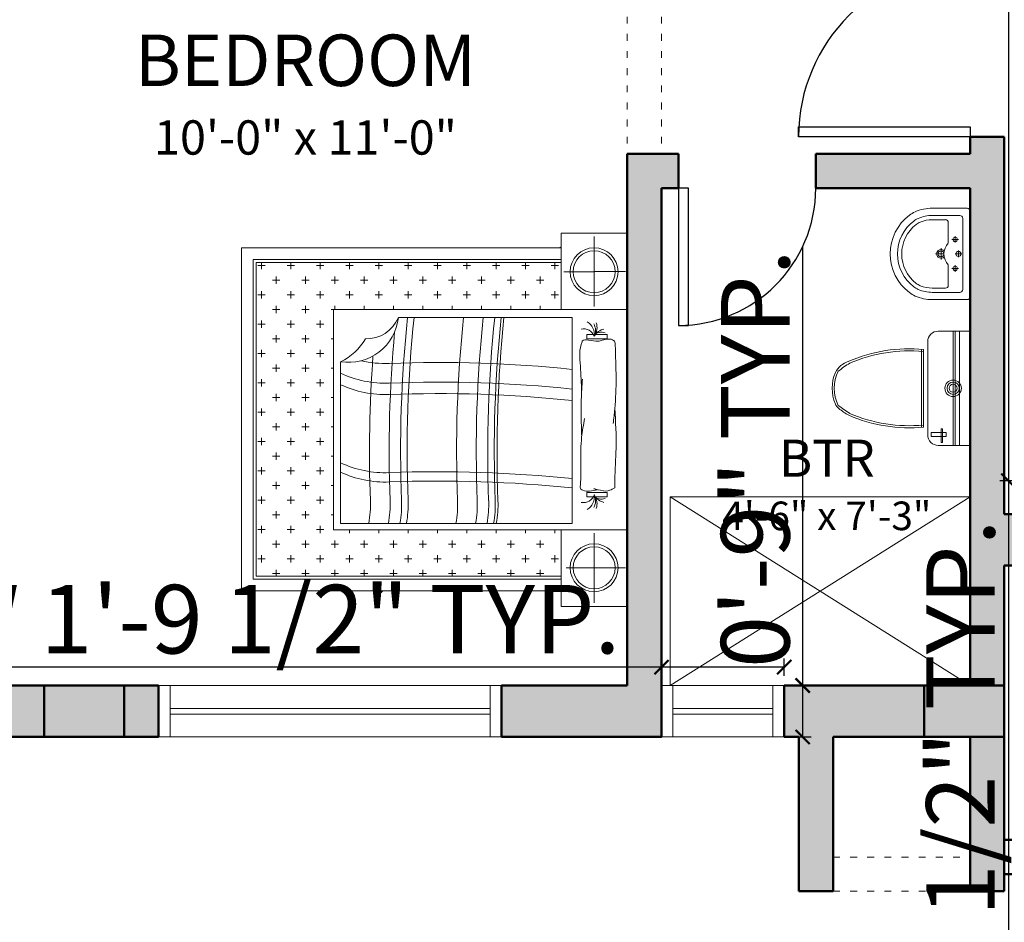
# Model space of a CAD drawing. Units: inches. Extents: x 375 to 1122, y 27 to 1069.
# Tile 3 of 155: x 494 to 667, y 155 to 313. Entities that reach past the tile are written whole.
import ezdxf

# ---------------------------------------------------------------- set-up
doc = ezdxf.new("R2010")
doc.units = ezdxf.units.IN
doc.linetypes.add('ACAD_ISO03W100', pattern=[30, 12, -18])
for name, color, linetype, lineweight in [('A-ANNO-DIMS', 2, 'Continuous', 18), ('A-AREA-IDEN', 7, 'Continuous', 18), ('A-COLS-PATT', 10, 'Continuous', 13), ('A-FLOR-FIXT', 55, 'Continuous', 18), ('A-WALL-OVHD', 77, 'ACAD_ISO03W100', 18), ('A-WALL-PATT', 252, 'Continuous', 13), ('Columns', 10, 'Continuous', 50), ('Doors', 150, 'Continuous', 25), ('Furniture', 30, 'Continuous', 18), ('Shower Areas', 53, 'Continuous', 18), ('Walls', 250, 'Continuous', 50), ('Windows', 122, 'Continuous', 18)]:
    doc.layers.add(name, color=color, linetype=linetype, lineweight=lineweight)
doc.styles.get("Standard").update_dxf_attribs({"font": 'arial.ttf'})
doc.dimstyles.new('ISO-25', dxfattribs={"dimtxt": 12, "dimasz": 2.5, "dimexe": 1.5, "dimexo": 1.5, "dimtad": 1, "dimdec": 1, "dimlunit": 3, "dimtxsty": 'Standard', "dimblk": 'ARCHTICK', "dimcen": 2.5, "dimadec": 0, "dimazin": 0, "dimtfac": 1, "dimtdec": 1, "dimtmove": 0, "dimatfit": 3, "dimfxl": 1.5, "dimfxlon": 1, "dimarcsym": 0})

# ---------------------------------------------------------------- blocks, each defined once
blk = doc.blocks.new('*U6')
for p, q in [((0, 0), (0, 4)), ((24, 0), (24, 4))]:
    blk.add_line(p, q)
blk.add_lwpolyline([(0, 0), (0, -24), (1.75, -24), (1.75, 0)], close=True)
blk.add_arc((0, 0), 24, 270, 0)
blk = doc.blocks.new('*U10')
for p, q in [((-30, 0), (-30, 4)), ((0, 0), (0, 4))]:
    blk.add_line(p, q)
blk.add_lwpolyline([(0, 0), (0, -30), (-1.75, -30), (-1.75, 0)], close=True)
blk.add_arc((0, 0), 30, 180, 270)
blk = doc.blocks.new('A$C52B64FF5')
for p, q in [((0.5216, 2.6276), (0, 2.6276)), ((0, 2.6276), (0, 2.1776)), ((0.5216, 2.1776), (0.5216, 2.6276)), ((2.0216, 2.6276), (0.5216, 2.6276)), ((0.5216, 2.6276), (0.5216, 0.6276)), ((2.5432, 2.6276), (2.0216, 2.6276)), ((2.0216, 0.6276), (2.0216, 2.6276)), ((2.0216, 2.6276), (2.0216, 2.1776)), ((2.5432, 2.1776), (2.5432, 2.6276)), ((0.2616, 2.4026), (0.2616, 2.6161)), ((2.2816, 2.4026), (2.2816, 2.6161)), ((0.721, 2.4927), (0.6917, 2.4927)), ((0.6917, 2.4927), (0.6917, 2.3531)), ((0.721, 2.3531), (0.721, 2.4927)), ((1.767, 2.3531), (1.767, 2.4927)), ((1.767, 2.4927), (1.7964, 2.4927)), ((1.7964, 2.4927), (1.7964, 2.3531)), ((0.2632, 2.4026), (0.0233, 2.4026)), ((0.0233, 2.4026), (0.4999, 2.4026)), ((0.2632, 2.1952), (0.2632, 2.4026)), ((0.6917, 2.3531), (0.721, 2.3531)), ((1.7964, 2.3531), (1.767, 2.3531)), ((2.5199, 2.4026), (2.0434, 2.4026)), ((2.2801, 2.2128), (2.2801, 2.4026)), ((2.2801, 2.4026), (2.5199, 2.4026)), ((0.5751, 1.0685), (0.5751, 2.2541)), ((0.5751, 2.2541), (1.9782, 2.2541)), ((1.9782, 2.2541), (1.9782, 0.6749)), ((0, 2.1776), (0.5216, 2.1776)), ((0.093, 2.1776), (0.1008, 2.1698)), ((0.1008, 0), (0.1008, 2.1776)), ((0.1808, 0.08), (0.1808, 2.1776)), ((0.2008, 0.1), (0.2008, 2.1776)), ((0.2197, 2.111), (0.2197, 2.161)), ((0.4197, 2.111), (0.4197, 2.161)), ((2.5432, 2.1776), (2.0216, 2.1776)), ((2.0216, 2.1776), (2.5432, 2.1776)), ((2.2197, 2.111), (2.2197, 2.161)), ((2.3374, 2.1776), (2.3374, 0.1)), ((2.3574, 2.1776), (2.3574, 0.08)), ((2.4374, 2.1776), (2.4374, 0)), ((0.2008, 2.136), (0.2447, 2.136)), ((0.3947, 2.136), (0.4447, 2.136)), ((2.0216, 2.136), (2.0447, 2.136)), ((2.1947, 2.136), (2.2447, 2.136)), ((0.2947, 2.036), (0.3447, 2.036)), ((0.3197, 2.011), (0.3197, 2.061)), ((0.4947, 2.036), (0.5216, 2.036)), ((0.5197, 2.011), (0.5197, 2.061)), ((2.0947, 2.036), (2.1447, 2.036)), ((2.1197, 2.011), (2.1197, 2.061)), ((2.2947, 2.036), (2.3374, 2.036)), ((2.3197, 2.011), (2.3197, 2.061)), ((0.2197, 1.911), (0.2197, 1.961)), ((0.4197, 1.911), (0.4197, 1.961)), ((2.2197, 1.911), (2.2197, 1.961)), ((0.2008, 1.936), (0.2447, 1.936)), ((0.3947, 1.936), (0.4447, 1.936)), ((2.0216, 1.936), (2.0447, 1.936)), ((2.1947, 1.936), (2.2447, 1.936)), ((0.2947, 1.836), (0.3447, 1.836)), ((0.3197, 1.811), (0.3197, 1.861)), ((0.4947, 1.836), (0.5216, 1.836)), ((0.5197, 1.811), (0.5197, 1.861)), ((2.0947, 1.836), (2.1447, 1.836)), ((2.1197, 1.811), (2.1197, 1.861)), ((2.2947, 1.836), (2.3374, 1.836)), ((2.3197, 1.811), (2.3197, 1.861)), ((0.2197, 1.711), (0.2197, 1.761)), ((0.4197, 1.711), (0.4197, 1.761)), ((2.2197, 1.711), (2.2197, 1.761)), ((0.2008, 1.736), (0.2447, 1.736)), ((0.3947, 1.736), (0.4447, 1.736)), ((2.0216, 1.736), (2.0447, 1.736)), ((2.1947, 1.736), (2.2447, 1.736)), ((0.2947, 1.636), (0.3447, 1.636)), ((0.3197, 1.611), (0.3197, 1.661)), ((0.4947, 1.636), (0.5216, 1.636)), ((0.5197, 1.611), (0.5197, 1.661)), ((2.0947, 1.636), (2.1447, 1.636)), ((2.1197, 1.611), (2.1197, 1.661)), ((2.2947, 1.636), (2.3374, 1.636)), ((2.3197, 1.611), (2.3197, 1.661)), ((0.2197, 1.511), (0.2197, 1.561)), ((0.4197, 1.511), (0.4197, 1.561)), ((2.2197, 1.511), (2.2197, 1.561)), ((0.2008, 1.536), (0.2447, 1.536)), ((0.3947, 1.536), (0.4447, 1.536)), ((2.0216, 1.536), (2.0447, 1.536)), ((2.1947, 1.536), (2.2447, 1.536)), ((0.2947, 1.436), (0.3447, 1.436)), ((0.3197, 1.411), (0.3197, 1.461)), ((0.4947, 1.436), (0.5216, 1.436)), ((0.5197, 1.411), (0.5197, 1.461)), ((2.0947, 1.436), (2.1447, 1.436)), ((2.1197, 1.411), (2.1197, 1.461)), ((2.2947, 1.436), (2.3374, 1.436)), ((2.3197, 1.411), (2.3197, 1.461)), ((0.2197, 1.311), (0.2197, 1.361)), ((0.4197, 1.311), (0.4197, 1.361)), ((2.2197, 1.311), (2.2197, 1.361)), ((0.2008, 1.336), (0.2447, 1.336)), ((0.3947, 1.336), (0.4447, 1.336)), ((2.0216, 1.336), (2.0447, 1.336)), ((2.1947, 1.336), (2.2447, 1.336)), ((0.2947, 1.236), (0.3447, 1.236)), ((0.3197, 1.211), (0.3197, 1.261)), ((0.4947, 1.236), (0.5216, 1.236)), ((0.5197, 1.211), (0.5197, 1.261)), ((2.0947, 1.236), (2.1447, 1.236)), ((2.1197, 1.211), (2.1197, 1.261)), ((2.2947, 1.236), (2.3374, 1.236)), ((2.3197, 1.211), (2.3197, 1.261)), ((0.2197, 1.111), (0.2197, 1.161)), ((0.4197, 1.111), (0.4197, 1.161)), ((2.2197, 1.111), (2.2197, 1.161)), ((0.2008, 1.136), (0.2447, 1.136)), ((0.3947, 1.136), (0.4447, 1.136)), ((2.0216, 1.136), (2.0447, 1.136)), ((2.1947, 1.136), (2.2447, 1.136)), ((0.2947, 1.036), (0.3447, 1.036)), ((0.3197, 1.011), (0.3197, 1.061)), ((0.4947, 1.036), (0.5216, 1.036)), ((0.5197, 1.011), (0.5197, 1.061)), ((2.0947, 1.036), (2.1447, 1.036)), ((2.1197, 1.011), (2.1197, 1.061)), ((2.2947, 1.036), (2.3374, 1.036)), ((2.3197, 1.011), (2.3197, 1.061)), ((0.2197, 0.911), (0.2197, 0.961)), ((0.4197, 0.911), (0.4197, 0.961)), ((2.2197, 0.911), (2.2197, 0.961)), ((2.4374, 0.9617), (2.4642, 0.935)), ((0.2008, 0.936), (0.2447, 0.936)), ((0.3947, 0.936), (0.4447, 0.936)), ((2.0216, 0.936), (2.0447, 0.936)), ((2.1947, 0.936), (2.2447, 0.936)), ((0.2947, 0.836), (0.3447, 0.836)), ((0.3197, 0.811), (0.3197, 0.861)), ((0.4947, 0.836), (0.5216, 0.836)), ((0.5197, 0.811), (0.5197, 0.861)), ((2.0947, 0.836), (2.1447, 0.836)), ((2.1197, 0.811), (2.1197, 0.861)), ((2.2947, 0.836), (2.3374, 0.836)), ((2.3197, 0.811), (2.3197, 0.861)), ((0.2197, 0.711), (0.2197, 0.761)), ((0.4197, 0.711), (0.4197, 0.761)), ((2.2197, 0.711), (2.2197, 0.761)), ((0.2008, 0.736), (0.2447, 0.736)), ((0.3947, 0.736), (0.4447, 0.736)), ((1.9782, 0.6749), (0.8764, 0.6749)), ((2.0216, 0.736), (2.0447, 0.736)), ((2.1947, 0.736), (2.2447, 0.736)), ((0.2947, 0.636), (0.3447, 0.636)), ((0.3197, 0.611), (0.3197, 0.661)), ((0.4947, 0.636), (0.5216, 0.636)), ((0.5197, 0.611), (0.5197, 0.661)), ((0.5216, 0.6276), (2.0216, 0.6276)), ((0.7197, 0.611), (0.7197, 0.6276)), ((0.9197, 0.611), (0.9197, 0.6276)), ((1.1197, 0.611), (1.1197, 0.6276)), ((1.3197, 0.611), (1.3197, 0.6276)), ((1.5197, 0.611), (1.5197, 0.6276)), ((1.7197, 0.611), (1.7197, 0.6276)), ((1.9197, 0.611), (1.9197, 0.6276)), ((2.0947, 0.636), (2.1447, 0.636)), ((2.1197, 0.611), (2.1197, 0.661)), ((2.2947, 0.636), (2.3374, 0.636)), ((2.3197, 0.611), (2.3197, 0.661)), ((0.2197, 0.511), (0.2197, 0.561)), ((0.4197, 0.511), (0.4197, 0.561)), ((0.6197, 0.511), (0.6197, 0.561)), ((0.8197, 0.511), (0.8197, 0.561)), ((1.0197, 0.511), (1.0197, 0.561)), ((1.2197, 0.511), (1.2197, 0.561)), ((1.4197, 0.511), (1.4197, 0.561)), ((1.6197, 0.511), (1.6197, 0.561)), ((1.8197, 0.511), (1.8197, 0.561)), ((2.0197, 0.511), (2.0197, 0.561)), ((2.2197, 0.511), (2.2197, 0.561)), ((0.2008, 0.536), (0.2447, 0.536)), ((0.3947, 0.536), (0.4447, 0.536)), ((0.5947, 0.536), (0.6447, 0.536)), ((0.7947, 0.536), (0.8447, 0.536)), ((0.9947, 0.536), (1.0447, 0.536)), ((1.1947, 0.536), (1.2447, 0.536)), ((1.3947, 0.536), (1.4447, 0.536)), ((1.5947, 0.536), (1.6447, 0.536)), ((1.7947, 0.536), (1.8447, 0.536)), ((1.9947, 0.536), (2.0447, 0.536)), ((2.1947, 0.536), (2.2447, 0.536)), ((0.2947, 0.436), (0.3447, 0.436)), ((0.3197, 0.411), (0.3197, 0.461)), ((0.4947, 0.436), (0.5447, 0.436)), ((0.5197, 0.411), (0.5197, 0.461)), ((0.6947, 0.436), (0.7447, 0.436)), ((0.7197, 0.411), (0.7197, 0.461)), ((0.8947, 0.436), (0.9447, 0.436)), ((0.9197, 0.411), (0.9197, 0.461)), ((1.0947, 0.436), (1.1447, 0.436)), ((1.1197, 0.411), (1.1197, 0.461)), ((1.2947, 0.436), (1.3447, 0.436)), ((1.3197, 0.411), (1.3197, 0.461)), ((1.4947, 0.436), (1.5447, 0.436)), ((1.5197, 0.411), (1.5197, 0.461)), ((1.6947, 0.436), (1.7447, 0.436)), ((1.7197, 0.411), (1.7197, 0.461)), ((1.8947, 0.436), (1.9447, 0.436)), ((1.9197, 0.411), (1.9197, 0.461)), ((2.0947, 0.436), (2.1447, 0.436)), ((2.1197, 0.411), (2.1197, 0.461)), ((2.2947, 0.436), (2.3374, 0.436)), ((2.3197, 0.411), (2.3197, 0.461)), ((0.2008, 0.336), (0.2447, 0.336)), ((0.2197, 0.311), (0.2197, 0.361)), ((0.3947, 0.336), (0.4447, 0.336)), ((0.4197, 0.311), (0.4197, 0.361)), ((0.5947, 0.336), (0.6447, 0.336)), ((0.6197, 0.311), (0.6197, 0.361)), ((0.7947, 0.336), (0.8447, 0.336)), ((0.8197, 0.311), (0.8197, 0.361)), ((0.9947, 0.336), (1.0447, 0.336)), ((1.0197, 0.311), (1.0197, 0.361)), ((1.1947, 0.336), (1.2447, 0.336)), ((1.2197, 0.311), (1.2197, 0.361)), ((1.3947, 0.336), (1.4447, 0.336)), ((1.4197, 0.311), (1.4197, 0.361)), ((1.5947, 0.336), (1.6447, 0.336)), ((1.6197, 0.311), (1.6197, 0.361)), ((1.7947, 0.336), (1.8447, 0.336)), ((1.8197, 0.311), (1.8197, 0.361)), ((1.9947, 0.336), (2.0447, 0.336)), ((2.0197, 0.311), (2.0197, 0.361)), ((2.1947, 0.336), (2.2447, 0.336)), ((2.2197, 0.311), (2.2197, 0.361)), ((0.2947, 0.236), (0.3447, 0.236)), ((0.3197, 0.211), (0.3197, 0.261)), ((0.4947, 0.236), (0.5447, 0.236)), ((0.5197, 0.211), (0.5197, 0.261)), ((0.6947, 0.236), (0.7447, 0.236)), ((0.7197, 0.211), (0.7197, 0.261)), ((0.8947, 0.236), (0.9447, 0.236)), ((0.9197, 0.211), (0.9197, 0.261)), ((1.0947, 0.236), (1.1447, 0.236)), ((1.1197, 0.211), (1.1197, 0.261)), ((1.2947, 0.236), (1.3447, 0.236)), ((1.3197, 0.211), (1.3197, 0.261)), ((1.4947, 0.236), (1.5447, 0.236)), ((1.5197, 0.211), (1.5197, 0.261)), ((1.6947, 0.236), (1.7447, 0.236)), ((1.7197, 0.211), (1.7197, 0.261)), ((1.8947, 0.236), (1.9447, 0.236)), ((1.9197, 0.211), (1.9197, 0.261)), ((2.0947, 0.236), (2.1447, 0.236)), ((2.1197, 0.211), (2.1197, 0.261)), ((2.2947, 0.236), (2.3374, 0.236)), ((2.3197, 0.211), (2.3197, 0.261)), ((0.2008, 0.136), (0.2447, 0.136)), ((0.2197, 0.111), (0.2197, 0.161)), ((0.3947, 0.136), (0.4447, 0.136)), ((0.4197, 0.111), (0.4197, 0.161)), ((0.5947, 0.136), (0.6447, 0.136)), ((0.6197, 0.111), (0.6197, 0.161)), ((0.7947, 0.136), (0.8447, 0.136)), ((0.8197, 0.111), (0.8197, 0.161)), ((0.9947, 0.136), (1.0447, 0.136)), ((1.0197, 0.111), (1.0197, 0.161)), ((1.1947, 0.136), (1.2447, 0.136)), ((1.2197, 0.111), (1.2197, 0.161)), ((1.3947, 0.136), (1.4447, 0.136)), ((1.4197, 0.111), (1.4197, 0.161)), ((1.5947, 0.136), (1.6447, 0.136)), ((1.6197, 0.111), (1.6197, 0.161)), ((1.7947, 0.136), (1.8447, 0.136)), ((1.8197, 0.111), (1.8197, 0.161)), ((1.9947, 0.136), (2.0447, 0.136)), ((2.0197, 0.111), (2.0197, 0.161)), ((2.1947, 0.136), (2.2447, 0.136)), ((2.2197, 0.111), (2.2197, 0.161)), ((2.3574, 0.08), (0.1808, 0.08)), ((2.3374, 0.1), (0.2008, 0.1)), ((2.4374, 0), (0.1008, 0))]:
    blk.add_line(p, q)
for centre, radius in [((0.2632, 2.4026), 0.1631), ((2.2801, 2.4026), 0.1631), ((0.2632, 2.4026), 0.1431), ((2.2801, 2.4026), 0.1431)]:
    blk.add_circle(centre, radius)
for centre, radius, start, end in [((0.6442, 2.3154), 0.1072, 59.2174, 107.24009), ((0.7523, 2.4916), 0.1013, 192.77399, 239.2386), ((0.7566, 2.4523), 0.0808, 161.45592, 221.5545), ((1.7358, 2.4916), 0.1013, 300.7614, 347.22601), ((1.8439, 2.3154), 0.1072, 72.75991, 120.7826), ((1.7315, 2.4523), 0.0808, 318.4455, 18.54408), ((0.6895, 2.3063), 0.098, 80.94857, 149.48786), ((0.6646, 2.3215), 0.0913, 67.83977, 120.48585), ((0.7294, 2.33), 0.0776, 109.26419, 192.26691), ((1.7587, 2.33), 0.0776, 347.73309, 73.88358), ((1.7986, 2.3063), 0.098, 30.51214, 99.05143), ((1.8235, 2.3215), 0.0913, 59.51415, 112.16023), ((9.7293, 1.3409), 8.8479, 174.07538, 182.16616), ((9.8633, 1.3409), 8.8479, 174.07538, 182.16616), ((9.9414, 1.3409), 8.8479, 174.07538, 182.16616), ((10.4736, 1.3409), 8.8479, 174.07538, 182.16616), ((10.5369, 1.3409), 8.8479, 174.07538, 182.16616), ((1.4884, 10.5889), 8.8479, 264.07538, 272.16616), ((1.4884, 10.5702), 8.8479, 264.07538, 272.16616), ((1.85, 1.0282), 0.7196, 79.7409, 92.16616), ((1.4884, 10.5256), 8.8479, 264.07538, 272.16616), ((1.85, 1.0096), 0.7196, 79.7409, 92.16616), ((1.85, 0.965), 0.7196, 79.7409, 92.16616), ((1.4884, 10.4474), 8.8479, 264.07538, 272.16616), ((1.85, 0.8868), 0.7196, 79.7409, 92.16616), ((1.4884, 10.3135), 8.8479, 264.07538, 272.16616), ((1.85, 0.7528), 0.7196, 79.7409, 92.16616), ((1.4884, 9.9764), 8.8479, 264.07538, 272.16616), ((1.4884, 9.9317), 8.8479, 264.07538, 272.16616), ((1.85, 0.4158), 0.7196, 79.7409, 92.16616), ((1.85, 0.3711), 0.7196, 79.7409, 92.16616), ((0.4865, 0.8516), 0.2343, 358.03681, 67.7864), ((0.5391, 0.7288), 0.3416, 350.92672, 83.95649), ((1.4884, 9.8536), 8.8479, 264.70583, 272.16616), ((1.85, 0.293), 0.7196, 79.7409, 92.16616), ((0.1687, 0.9792), 0.7196, 346.86533, 2.16616), ((0.3027, 0.9792), 0.7196, 334.98359, 2.16616), ((0.3808, 0.9792), 0.7196, 334.98359, 2.16616), ((0.913, 0.9792), 0.7196, 334.98359, 2.16616), ((0.9763, 0.9792), 0.7196, 334.98359, 2.16616), ((1.4884, 9.7196), 8.8479, 265.77852, 272.16616), ((1.85, 0.159), 0.7196, 79.7409, 92.16616), ((0.5285, 0.5098), 0.3852, 25.3912, 60.06861)]:
    blk.add_arc(centre, radius, start, end)
for points, knots in [([(0.7373, 2.4293), (0.7344, 2.4386), (0.7239, 2.472), (0.715, 2.518), (0.7414, 2.5459), (0.9088, 2.5514), (1.0864, 2.5586), (1.2642, 2.5365), (1.2976, 2.5323)], [0, 0, 0, 0, 0.0298664, 0.1071619, 0.1152509, 0.1416099, 0.5761797, 0.6768951, 0.6768951, 0.6768951, 0.6768951]), ([(1.1947, 2.5438), (1.2853, 2.549), (1.4483, 2.5585), (1.6283, 2.5432), (1.7179, 2.5437), (1.7351, 2.5438)], [0, 0, 0, 0, 0.2717358, 0.4891854, 0.5406465, 0.5406465, 0.5406465, 0.5406465]), ([(1.7351, 2.5438), (1.7416, 2.5321), (1.759, 2.5014), (1.7583, 2.4623), (1.7348, 2.3817), (1.7455, 2.4145), (1.7494, 2.4265)], [0, 0, 0, 0, 0.0383771, 0.1013156, 0.1484959, 0.1756343, 0.1756343, 0.1756343, 0.1756343]), ([(1.0802, 2.3175), (1.0225, 2.3155), (0.9099, 2.3116), (0.7905, 2.2985), (0.7234, 2.3279), (0.7309, 2.3766), (0.7348, 2.4091), (0.7373, 2.4293)], [0, 0, 0, 0, 0.1744349, 0.3406483, 0.347042, 0.3874998, 0.4538558, 0.4538558, 0.4538558, 0.4538558]), ([(1.7494, 2.4265), (1.7531, 2.4084), (1.7601, 2.3751), (1.7573, 2.3363), (1.7437, 2.3065), (1.6676, 2.315), (1.559, 2.3108), (1.4028, 2.3119), (1.305, 2.3301), (1.2633, 2.3378)], [0, 0, 0, 0, 0.0550284, 0.1011576, 0.1178362, 0.1437253, 0.3009935, 0.4726259, 0.6000038, 0.6000038, 0.6000038, 0.6000038]), ([(1.3748, 2.3178), (1.2947, 2.315), (1.1678, 2.3105), (1.0413, 2.32), (0.9946, 2.3235)], [0, 0, 0, 0, 0.2401688, 0.38052, 0.38052, 0.38052, 0.38052])]:
    blk.add_open_spline(points, degree=3, knots=knots)
blk = doc.blocks.new('A$C00C51FE0')
at = {"ltscale": 2}
for p, q in [((1.85, 7.41), (18.15, 7.41)), ((16.79, 8.49), (3.21, 8.49)), ((16.79, 8.12), (3.21, 8.12)), ((0, 0), (0, 5.56)), ((1.59, 4.18), (1.59, 6.81)), ((1.59, 6.81), (2.25, 6.81)), ((2.25, 6.81), (2.25, 4.18)), ((20, 5.56), (20, 0)), ((0.5, 4.84), (0.5, 5.06)), ((0.5, 5.06), (2.91, 5.06)), ((2.91, 4.84), (0.5, 4.84)), ((2.25, 4.18), (1.59, 4.18)), ((2.91, 5.06), (2.91, 4.84)), ((20, 2.96), (0, 2.96)), ((20, 2.59), (0, 2.59)), ((20, 1.85), (0, 1.85)), ((20, 0), (0, 0))]:
    blk.add_line(p, q, dxfattribs=at)
for radius in [1.44, 1.07, 0.698]:
    blk.add_circle((10, 2.96), radius, dxfattribs=at)
for centre, radius, start, end in [((10, 17.03), 7.1, 67.0801, 112.9199), ((22.68, 10.69), 20.34, 142.816, 148.8373), ((22.68, 10.69), 19.97, 141.7352, 148.8373), ((7.96, 21.86), 1.85, 112.9199, 142.816), ((10, 17.03), 6.73, 63.5839, 116.4161), ((11.04, 20.15), 3.83, 16.1902, 63.2078), ((-2.68, 10.69), 19.97, 31.1627, 38.2648), ((29.69, 10.65), 26.6, 156.5869, 185.4494), ((29.69, 10.65), 26.23, 156.5869, 185.4494), ((-9.69, 10.65), 26.23, 354.5506, 23.4131), ((-9.69, 10.65), 26.6, 354.5506, 23.4131), ((1.85, 5.56), 1.85, 90, 180), ((18.15, 5.56), 1.85, 0, 90)]:
    blk.add_arc(centre, radius, start, end, dxfattribs=at)
blk = doc.blocks.new('WINDOW-21_5IN')
for p, q in [((4, 2), (4, 19.5)), ((5, 2), (5, 19.5))]:
    blk.add_line(p, q)
blk.add_lwpolyline([(0, 0), (9, 0), (9, 21.5), (0, 21.5)], close=True)
for points in [[(9, 19.5), (0, 19.5)], [(0, 2), (9, 2)]]:
    blk.add_lwpolyline(points)
blk = doc.blocks.new('WINDOW-60IN')
for p, q in [((58, 5), (2, 5)), ((58, 4), (2, 4))]:
    blk.add_line(p, q)
blk.add_lwpolyline([(60, 0), (0, 0), (0, 9), (60, 9)], close=True)
for points in [[(2, 0), (2, 9)], [(58, 9), (58, 0)]]:
    blk.add_lwpolyline(points)
blk = doc.blocks.new('LAVATORY-16IN')
for p, q in [((1.27, 7.37), (1.27, 12.19)), ((1.78, 12.7), (14.22, 12.7)), ((8, 11.37), (8, 12.51)), ((14.73, 12.19), (14.73, 7.37)), ((4.89, 11.37), (6.03, 11.37)), ((5.46, 10.79), (5.46, 11.94)), ((7.43, 11.94), (8.57, 11.94)), ((9.97, 11.37), (11.11, 11.37)), ((10.54, 10.79), (10.54, 11.94)), ((2.01, 7.37), (2.01, 9.65)), ((2.51, 10.16), (6.08, 10.16)), ((7.02, 8.89), (8.98, 8.89)), ((8, 7.91), (8, 9.4)), ((9.91, 10.16), (13.49, 10.16)), ((13.99, 9.65), (13.99, 7.37))]:
    blk.add_line(p, q)
blk.add_lwpolyline([(0.51, 13.97), (15.49, 13.97, -0.414214), (16, 13.46), (16, 7.37, -0.104704), (15.37, 4.36, -0.038376), (14.78, 3.36, -0.495903), (1.22, 3.36, -0.038376), (0.63, 4.36, -0.104704), (0, 7.37), (0, 13.46, -0.414214)], format="xyb", close=True)
for points in [[(1.27, 7.37, 0.102694), (1.78, 4.92, 0.037256), (2.25, 4.11, 0.085618)], [(2.01, 7.37, 0.101044), (2.44, 5.24, 0.036381), (2.84, 4.54, 0.084644)], [(13.16, 4.54, 0.036381), (13.56, 5.24, 0.101044), (13.99, 7.37, 0.11083)], [(13.75, 4.11, 0.037256), (14.22, 4.92, 0.102694), (14.73, 7.37, 0.111333)]]:
    blk.add_lwpolyline(points, format="xyb")
for centre, radius in [((8, 11.94), 0.444), ((5.46, 11.37), 0.381), ((10.54, 11.37), 0.381), ((8, 8.89), 0.508)]:
    blk.add_circle(centre, radius)
for centre, radius, start, end in [((1.78, 12.19), 0.508, 90, 180), ((14.22, 12.19), 0.508, 0, 90), ((2.51, 9.65), 0.508, 90, 180), ((7.99, 12.19), 2.79, 226.6581, 313.3419), ((8, 8.89), 0.762, 133.135, 47.0367), ((13.49, 9.65), 0.508, 0, 90), ((8, 8.52), 7.25, 217.471, 322.529), ((8, 8.52), 6.51, 217.6433, 322.3567)]:
    blk.add_arc(centre, radius, start, end)
blk = doc.blocks.new('COLUMN-14X9IN')
blk.add_lwpolyline([(0, 0), (14, 0), (14, 9), (0, 9)], close=True)
blk = doc.blocks.new('SHOWER-PAN-52_5X33IN')
for p, q in [((0, 33), (52.5, 0)), ((52.5, 33), (0, 0))]:
    blk.add_line(p, q)
blk.add_lwpolyline([(0, 0), (52.5, 0), (52.5, 33), (0, 33)], close=True)
blk = doc.blocks.new('_ArchTick')
at = {"color": 0, "linetype": 'ByBlock', "const_width": 0.15}
blk.add_lwpolyline([(-0.5, -0.5), (0.5, 0.5)], dxfattribs=at)
blk = doc.blocks.new('*D49')
at = {"layer": 'A-ANNO-DIMS', "color": 0, "lineweight": -2, "transparency": 16777216}
for p, q in [((606.51, 198.25), (606.51, 201.25)), ((628.01, 198.25), (628.01, 201.25)), ((606.51, 199.75), (374.6, 199.75)), ((628.01, 199.75), (606.51, 199.75))]:
    blk.add_line(p, q, dxfattribs=at)
at = {"layer": 'Defpoints', "color": 0, "transparency": 16777216}
for p in [(606.51, 199.75), (606.51, 196.53), (628.01, 196.53)]:
    blk.add_point(p, dxfattribs=at)
at = {"layer": 'A-ANNO-DIMS', "color": 0, "lineweight": -2, "transparency": 16777216, "xscale": 2.5, "yscale": 2.5, "zscale": 2.5, "rotation": 180}
blk.add_blockref('_ArchTick', (606.51, 199.75), dxfattribs=at)
at = {"layer": 'A-ANNO-DIMS', "color": 0, "lineweight": -2, "transparency": 16777216, "xscale": 2.5, "yscale": 2.5, "zscale": 2.5}
blk.add_blockref('_ArchTick', (628.01, 199.75), dxfattribs=at)
at = {"layer": 'A-ANNO-DIMS', "color": 0, "transparency": 16777216, "insert": (489.3, 206.59), "char_height": 12, "attachment_point": 5}
blk.add_mtext('BATH WINDOW 1\'-9 1/2" TYP.', dxfattribs=at)
blk = doc.blocks.new('*D50')
at = {"layer": 'A-ANNO-DIMS', "color": 0, "lineweight": -2, "transparency": 16777216}
for p, q in [((631.23, 196.53), (631.23, 273.42)), ((629.73, 196.53), (632.73, 196.53)), ((631.23, 187.53), (631.23, 196.53)), ((629.73, 187.53), (632.73, 187.53))]:
    blk.add_line(p, q, dxfattribs=at)
at = {"layer": 'Defpoints', "color": 0, "transparency": 16777216}
for p in [(628.01, 196.53), (631.23, 196.53), (628.01, 187.53)]:
    blk.add_point(p, dxfattribs=at)
at = {"layer": 'A-ANNO-DIMS', "color": 0, "lineweight": -2, "transparency": 16777216, "xscale": 2.5, "yscale": 2.5, "zscale": 2.5}
for p, rotation in [((631.23, 196.53), 90), ((631.23, 187.53), 270)]:
    blk.add_blockref('_ArchTick', p, dxfattribs=dict(at, rotation=rotation))
at = {"layer": 'A-ANNO-DIMS', "color": 0, "transparency": 16777216, "insert": (624.48, 236.23), "char_height": 12, "attachment_point": 5, "rotation": 90}
blk.add_mtext('0\'-9" TYP.', dxfattribs=at)
blk = doc.blocks.new('*D59')
at = {"layer": 'A-ANNO-DIMS', "color": 0, "lineweight": -2, "transparency": 16777216}
for p, q in [((668.72, 346.85), (665.72, 346.85)), ((667.22, 346.85), (667.22, 232.35)), ((668.72, 232.35), (665.72, 232.35)), ((667.22, 232.35), (667.22, 27.5))]:
    blk.add_line(p, q, dxfattribs=at)
at = {"layer": 'Defpoints', "color": 0, "transparency": 16777216}
for p in [(684.39, 346.85), (667.22, 232.35), (684.39, 232.35)]:
    blk.add_point(p, dxfattribs=at)
at = {"layer": 'A-ANNO-DIMS', "color": 0, "lineweight": -2, "transparency": 16777216, "xscale": 2.5, "yscale": 2.5, "zscale": 2.5}
for p, rotation in [((667.22, 346.85), 90), ((667.22, 232.35), 270)]:
    blk.add_blockref('_ArchTick', p, dxfattribs=dict(at, rotation=rotation))
at = {"layer": 'A-ANNO-DIMS', "color": 0, "transparency": 16777216, "insert": (660.39, 128.67), "char_height": 12, "attachment_point": 5, "rotation": 90}
blk.add_mtext('DINING SET 9\'-6 1/2" TYP.', dxfattribs=at)
blk = doc.blocks.new('*D81')
at = {"layer": 'A-ANNO-DIMS', "color": 0, "lineweight": -2, "transparency": 16777216}
for p, q in [((444.51, 117.53), (444.51, 114.53)), ((989.01, 117.53), (989.01, 114.53)), ((444.51, 116.03), (989.01, 116.03))]:
    blk.add_line(p, q, dxfattribs=at)
at = {"layer": 'Defpoints', "color": 0, "transparency": 16777216}
for p in [(444.51, 187.53), (989.01, 187.53), (989.01, 116.03)]:
    blk.add_point(p, dxfattribs=at)
at = {"layer": 'A-ANNO-DIMS', "color": 0, "lineweight": -2, "transparency": 16777216, "xscale": 2.5, "yscale": 2.5, "zscale": 2.5, "rotation": 180}
blk.add_blockref('_ArchTick', (444.51, 116.03), dxfattribs=at)
at = {"layer": 'A-ANNO-DIMS', "color": 0, "lineweight": -2, "transparency": 16777216, "xscale": 2.5, "yscale": 2.5, "zscale": 2.5}
blk.add_blockref('_ArchTick', (989.01, 116.03), dxfattribs=at)
at = {"layer": 'A-ANNO-DIMS', "color": 0, "transparency": 16777216, "insert": (716.76, 122.86), "char_height": 12, "attachment_point": 5}
blk.add_mtext('45\'-4 1/2"', dxfattribs=at)
blk = doc.blocks.new('*D82')
at = {"layer": 'A-ANNO-DIMS', "color": 0, "lineweight": -2, "transparency": 16777216}
for p, q in [((401.51, 1009.53), (398.51, 1009.53)), ((400.01, 160.53), (400.01, 1009.53)), ((401.51, 160.53), (398.51, 160.53))]:
    blk.add_line(p, q, dxfattribs=at)
at = {"layer": 'Defpoints', "color": 0, "transparency": 16777216}
for p in [(400.01, 1009.53), (630.53, 1009.53), (630.53, 160.53)]:
    blk.add_point(p, dxfattribs=at)
at = {"layer": 'A-ANNO-DIMS', "color": 0, "lineweight": -2, "transparency": 16777216, "xscale": 2.5, "yscale": 2.5, "zscale": 2.5}
for p, rotation in [((400.01, 1009.53), 90), ((400.01, 160.53), 270)]:
    blk.add_blockref('_ArchTick', p, dxfattribs=dict(at, rotation=rotation))
at = {"layer": 'A-ANNO-DIMS', "color": 0, "transparency": 16777216, "insert": (393.26, 585.03), "char_height": 12, "attachment_point": 5, "rotation": 90}
blk.add_mtext('70\'-9"', dxfattribs=at)

msp = doc.modelspace()

# ---------------------------------------------------------------- hatches: boundary and pattern name
at = {"layer": 'A-COLS-PATT'}
h = msp.add_hatch(color=256, dxfattribs=at)
h.dxf.hatch_style = 1
h.paths.add_polyline_path([(512.51, 982.53), (498.51, 982.53), (498.51, 973.53), (512.51, 973.53)])
h.paths.add_polyline_path([(666.51, 982.53), (652.51, 982.53), (652.51, 973.53), (666.51, 973.53)])
h.paths.add_polyline_path([(802.01, 982.53), (788.01, 982.53), (788.01, 973.53), (802.01, 973.53)])
h.paths.add_polyline_path([(932.01, 982.53), (918.01, 982.53), (918.01, 973.53), (932.01, 973.53)])
h.paths.add_polyline_path([(507.51, 841.53), (498.51, 841.53), (498.51, 827.53), (507.51, 827.53)])
h.paths.add_polyline_path([(666.51, 844.53), (652.51, 844.53), (652.51, 835.53), (666.51, 835.53)])
h.paths.add_polyline_path([(802.01, 814.53), (788.01, 814.53), (788.01, 805.53), (802.01, 805.53)])
h.paths.add_polyline_path([(932.01, 814.53), (918.01, 814.53), (918.01, 805.53), (932.01, 805.53)])
h.paths.add_polyline_path([(507.51, 719.53), (498.51, 719.53), (498.51, 705.53), (507.51, 705.53)])
h.paths.add_polyline_path([(731.01, 676.53), (722.01, 676.53), (722.01, 662.53), (731.01, 662.53)])
h.paths.add_polyline_path([(802.01, 676.53), (788.01, 676.53), (788.01, 667.53), (802.01, 667.53)])
h.paths.add_polyline_path([(932.01, 676.53), (918.01, 676.53), (918.01, 667.53), (932.01, 667.53)])
h.paths.add_polyline_path([(932.01, 583.53), (918.01, 583.53), (918.01, 574.53), (932.01, 574.53)])
h.paths.add_polyline_path([(868.01, 583.53), (854.01, 583.53), (854.01, 574.53), (868.01, 574.53)])
h.paths.add_polyline_path([(868.01, 502.53), (854.01, 502.53), (854.01, 493.53), (868.01, 493.53)])
h.paths.add_polyline_path([(932.01, 502.53), (918.01, 502.53), (918.01, 493.53), (932.01, 493.53)])
h.paths.add_polyline_path([(672.51, 592.03), (663.51, 592.03), (663.51, 578.03), (672.51, 578.03)])
h.paths.add_polyline_path([(512.51, 589.53), (498.51, 589.53), (498.51, 580.53), (512.51, 580.53)])
h.paths.add_polyline_path([(507.51, 464.53), (498.51, 464.53), (498.51, 450.53), (507.51, 450.53)])
h.paths.add_polyline_path([(731.01, 507.53), (722.01, 507.53), (722.01, 493.53), (731.01, 493.53)])
h.paths.add_polyline_path([(802.01, 502.53), (788.01, 502.53), (788.01, 493.53), (802.01, 493.53)])
h.paths.add_polyline_path([(507.51, 342.53), (498.51, 342.53), (498.51, 328.53), (507.51, 328.53)])
h.paths.add_polyline_path([(512.51, 196.53), (498.51, 196.53), (498.51, 187.53), (512.51, 187.53)])
h.paths.add_polyline_path([(666.51, 334.53), (652.51, 334.53), (652.51, 325.53), (666.51, 325.53)])
h.paths.add_polyline_path([(666.51, 196.53), (652.51, 196.53), (652.51, 187.53), (666.51, 187.53)])
h.paths.add_polyline_path([(805.01, 196.53), (791.01, 196.53), (791.01, 187.53), (805.01, 187.53)])
h.paths.add_polyline_path([(932.01, 196.53), (918.01, 196.53), (918.01, 187.53), (932.01, 187.53)])
h.paths.add_polyline_path([(932.01, 334.53), (918.01, 334.53), (918.01, 325.53), (932.01, 325.53)])
h.paths.add_polyline_path([(805.01, 334.53), (791.01, 334.53), (791.01, 325.53), (805.01, 325.53)])
at = {"layer": 'A-WALL-PATT'}
h = msp.add_hatch(color=256, dxfattribs=at)
h.dxf.hatch_style = 1
h.paths.add_polyline_path([(962.01, 388.53), (989.01, 388.53), (989.01, 394.53), (962.01, 394.53), (932.01, 394.53), (932.01, 397.53), (923.01, 397.53), (923.01, 394.53), (842.01, 394.53), (842.01, 334.53), (839.51, 334.53), (839.51, 328.53), (854.01, 328.53), (854.01, 334.53), (848.01, 334.53), (848.01, 388.53), (953.01, 388.53), (953.01, 356.08), (962.01, 356.08), (962.01, 358.55), (989.01, 358.55), (989.01, 364.55), (962.01, 364.55)])
h.paths.add_polyline_path([(989.01, 502.53), (932.01, 502.53), (932.01, 583.53), (932.01, 593.53), (923.01, 593.53), (923.01, 583.53), (854.01, 583.53), (854.01, 556.53), (863.01, 556.53), (863.01, 574.53), (923.01, 574.53), (923.01, 502.53), (863.01, 502.53), (863.01, 520.53), (854.01, 520.53), (854.01, 502.53), (773.01, 502.53), (773.01, 493.53), (788.01, 493.53), (788.01, 402.03), (722.01, 402.03), (722.01, 373.53), (728.01, 373.53), (728.01, 396.03), (788.01, 396.03), (788.01, 373.53), (794.01, 373.53), (794.01, 430.53), (814.01, 430.53), (814.01, 436.53), (794.01, 436.53), (794.01, 493.53), (923.01, 493.53), (923.01, 487.53), (932.01, 487.53), (932.01, 493.53), (983.01, 493.53), (983.01, 473.53), (989.01, 473.53)])
h.paths.add_polyline_path([(797.01, 325.53), (805.01, 325.53), (805.01, 328.53), (807.51, 328.53), (807.51, 334.53), (791.01, 334.53), (791.01, 226.53), (770.76, 226.53), (770.76, 217.53), (791.01, 217.53), (791.01, 187.53), (855.01, 187.53), (855.01, 196.53), (797.01, 196.53)])
h.paths.add_polyline_path([(989.01, 238.53), (962.01, 238.53), (962.01, 256.42), (953.01, 256.42), (953.01, 229.53), (980.01, 229.53), (980.01, 196.53), (915.01, 196.53), (915.01, 187.53), (989.01, 187.53)])
h.paths.add_polyline_path([(962.01, 334.53), (884.01, 334.53), (884.01, 328.53), (918.01, 328.53), (918.01, 325.53), (932.01, 325.53), (932.01, 328.53), (953.01, 328.53), (953.01, 304.42), (962.01, 304.42)])
h.paths.add_polyline_path([(606.51, 283.53), (609.51, 283.53), (609.51, 289.53), (600.51, 289.53), (600.51, 196.53), (578.51, 196.53), (578.51, 187.53), (606.51, 187.53), (606.51, 196.53)])
h.paths.add_polyline_path([(666.51, 292.53), (660.51, 292.53), (660.51, 289.53), (633.51, 289.53), (633.51, 283.53), (660.51, 283.53), (660.51, 196.53), (628.01, 196.53), (628.01, 187.53), (630.53, 187.53), (630.53, 160.53), (636.53, 160.53), (636.53, 187.53), (660.51, 187.53), (660.51, 160.53), (666.51, 160.53), (666.51, 217.53), (686.76, 217.53), (686.76, 226.53), (666.51, 226.53)])
h.paths.add_polyline_path([(480.51, 256.42), (471.51, 256.42), (471.51, 238.53), (444.51, 238.53), (444.51, 187.53), (518.51, 187.53), (518.51, 196.53), (453.51, 196.53), (453.51, 229.53), (480.51, 229.53)])
h.paths.add_polyline_path([(480.51, 328.53), (652.51, 328.53), (652.51, 325.53), (660.51, 325.53), (660.51, 322.53), (666.51, 322.53), (666.51, 334.53), (507.51, 334.53), (507.51, 360.53), (498.51, 360.53), (498.51, 334.53), (471.51, 334.53), (471.51, 304.42), (480.51, 304.42)])
h.paths.add_polyline_path([(507.51, 484.53), (498.51, 484.53), (498.51, 444.53), (507.51, 444.53), (507.51, 454.53), (621.51, 454.53), (621.51, 460.53), (507.51, 460.53)])
h.paths.add_polyline_path([(672.51, 604.53), (683.26, 604.53), (683.26, 613.53), (669.51, 613.53), (669.51, 649.53), (663.51, 649.53), (663.51, 589.53), (507.51, 589.53), (507.51, 613.53), (498.51, 613.53), (498.51, 556.53), (507.51, 556.53), (507.51, 580.53), (663.51, 580.53), (663.51, 520.53), (669.51, 520.53), (669.51, 556.53), (683.26, 556.53), (683.26, 565.53), (672.51, 565.53)])
h.paths.add_polyline_path([(731.01, 667.53), (734.01, 667.53), (734.01, 676.53), (728.01, 676.53), (728.01, 715.53), (657.51, 715.53), (657.51, 709.53), (663.51, 709.53), (663.51, 673.53), (669.51, 673.53), (669.51, 709.53), (722.01, 709.53), (722.01, 613.53), (704.76, 613.53), (704.76, 604.53), (722.01, 604.53), (722.01, 565.53), (704.76, 565.53), (704.76, 556.53), (722.01, 556.53), (722.01, 502.53), (722.01, 460.53), (669.51, 460.53), (669.51, 496.53), (663.51, 496.53), (663.51, 460.53), (657.51, 460.53), (657.51, 454.53), (728.01, 454.53), (728.01, 493.53), (734.01, 493.53), (734.01, 502.53), (731.01, 502.53)])
h.paths.add_polyline_path([(986.01, 718.53), (959.01, 718.53), (959.01, 727.53), (950.01, 727.53), (950.01, 709.53), (977.01, 709.53), (977.01, 676.53), (794.01, 676.53), (794.01, 805.53), (802.01, 805.53), (802.01, 808.53), (804.51, 808.53), (804.51, 814.53), (788.01, 814.53), (788.01, 774.03), (728.01, 774.03), (728.01, 796.53), (722.01, 796.53), (722.01, 768.03), (788.01, 768.03), (788.01, 676.53), (773.01, 676.53), (773.01, 667.53), (923.01, 667.53), (923.01, 657.53), (932.01, 657.53), (932.01, 667.53), (986.01, 667.53)])
h.paths.add_polyline_path([(621.51, 715.53), (507.51, 715.53), (507.51, 733.53), (498.51, 733.53), (498.51, 715.53), (498.51, 685.53), (507.51, 685.53), (507.51, 709.53), (621.51, 709.53)])
h.paths.add_polyline_path([(666.51, 847.03), (660.51, 847.03), (660.51, 844.53), (652.51, 844.53), (652.51, 841.53), (480.51, 841.53), (480.51, 859.53), (471.51, 859.53), (471.51, 835.53), (498.51, 835.53), (498.51, 817.53), (507.51, 817.53), (507.51, 835.53), (666.51, 835.53)])
h.paths.add_polyline_path([(480.51, 940.53), (453.51, 940.53), (453.51, 973.53), (518.51, 973.53), (518.51, 982.53), (444.51, 982.53), (444.51, 931.53), (471.51, 931.53), (471.51, 907.53), (480.51, 907.53)])
h.paths.add_polyline_path([(606.51, 982.53), (578.51, 982.53), (578.51, 973.53), (600.51, 973.53), (600.51, 880.53), (609.51, 880.53), (609.51, 886.53), (606.51, 886.53)])
h.paths.add_polyline_path([(666.51, 943.53), (686.76, 943.53), (686.76, 952.53), (666.51, 952.53), (666.51, 1009.53), (660.51, 1009.53), (660.51, 982.53), (636.53, 982.53), (636.53, 1009.53), (630.53, 1009.53), (630.53, 982.53), (628.01, 982.53), (628.01, 973.53), (660.51, 973.53), (660.51, 886.53), (633.51, 886.53), (633.51, 880.53), (660.51, 880.53), (660.51, 877.03), (666.51, 877.03)])
h.paths.add_polyline_path([(986.01, 874.53), (932.01, 874.53), (932.01, 877.53), (923.01, 877.53), (923.01, 874.53), (788.01, 874.53), (788.01, 868.53), (788.01, 844.53), (794.01, 844.53), (794.01, 868.53), (839.01, 868.53), (839.01, 814.53), (836.51, 814.53), (836.51, 808.53), (851.01, 808.53), (851.01, 814.53), (845.01, 814.53), (845.01, 868.53), (986.01, 868.53)])
h.paths.add_polyline_path([(959.01, 838.55), (986.01, 838.55), (986.01, 844.55), (959.01, 844.55), (959.01, 847.03), (950.01, 847.03), (950.01, 814.53), (881.01, 814.53), (881.01, 808.53), (918.01, 808.53), (918.01, 805.53), (932.01, 805.53), (932.01, 808.53), (950.01, 808.53), (950.01, 793.53), (959.01, 793.53)])
h.paths.add_polyline_path([(986.01, 982.53), (899.01, 982.53), (899.01, 973.53), (923.01, 973.53), (923.01, 967.53), (932.01, 967.53), (932.01, 973.53), (980.01, 973.53), (980.01, 953.53), (986.01, 953.53)])
h.paths.add_polyline_path([(851.01, 982.53), (788.01, 982.53), (788.01, 952.53), (770.76, 952.53), (770.76, 943.53), (788.01, 943.53), (788.01, 910.53), (814.01, 910.53), (814.01, 916.53), (794.01, 916.53), (794.01, 973.53), (851.01, 973.53)])

# ---------------------------------------------------------------- linework, layer by layer
at = {"layer": 'A-WALL-OVHD', "ltscale": 0.1}
for p, q in [((600.51, 328.53), (600.51, 289.53)), ((606.51, 328.53), (606.51, 289.53)), ((636.53, 166.53), (660.51, 166.53)), ((636.53, 160.53), (660.51, 160.53))]:
    msp.add_line(p, q, dxfattribs=at)
at = {"layer": 'Walls'}
for p, q in [((660.51, 292.53), (666.51, 292.53)), ((660.51, 292.53), (660.51, 289.53)), ((666.51, 292.53), (666.51, 226.53)), ((600.51, 289.53), (600.51, 196.53)), ((600.51, 289.53), (609.51, 289.53)), ((609.51, 283.53), (609.51, 289.53)), ((633.51, 283.53), (633.51, 289.53)), ((633.51, 289.53), (660.51, 289.53)), ((606.51, 283.53), (609.51, 283.53)), ((633.51, 283.53), (660.51, 283.53)), ((660.51, 283.53), (660.51, 196.53)), ((686.76, 226.53), (666.51, 226.53)), ((666.51, 217.53), (666.51, 160.53)), ((686.76, 217.53), (666.51, 217.53)), ((518.51, 196.53), (453.51, 196.53)), ((518.51, 187.53), (518.51, 196.53)), ((600.51, 196.53), (578.51, 196.53)), ((578.51, 187.53), (578.51, 196.53)), ((628.01, 196.53), (660.51, 196.53)), ((628.01, 196.53), (628.01, 187.53)), ((444.51, 187.53), (518.51, 187.53)), ((628.01, 187.53), (630.53, 187.53)), ((630.53, 187.53), (630.53, 160.53)), ((636.53, 160.53), (636.53, 187.53)), ((636.53, 187.53), (660.51, 187.53)), ((660.51, 160.53), (660.51, 187.53)), ((791.01, 169.53), (666.51, 169.53)), ((797.01, 163.53), (666.51, 163.53)), ((630.53, 160.53), (636.53, 160.53)), ((666.51, 160.53), (660.51, 160.53))]:
    msp.add_line(p, q, dxfattribs=at)
msp.add_lwpolyline([(606.51, 283.53), (606.51, 196.53), (606.51, 187.53), (578.51, 187.53)], dxfattribs=at)

# ---------------------------------------------------------------- block references
at = {"layer": 'A-FLOR-FIXT', "extrusion": (0, 0, -1), "zscale": -1, "rotation": 90}
msp.add_blockref('LAVATORY-16IN', (-646.54, 264.04), dxfattribs=at)
at = {"layer": 'A-FLOR-FIXT', "rotation": 89.99999999999999}
msp.add_blockref('A$C00C51FE0', (660.51, 238.53), dxfattribs=at)
at = {"layer": 'Columns', "rotation": 180}
for p in [(512.51, 196.53), (666.51, 196.53)]:
    msp.add_blockref('COLUMN-14X9IN', p, dxfattribs=at)
at = {"layer": 'Doors', "rotation": 270}
msp.add_blockref('*U10', (660.51, 292.53), dxfattribs=at)
at = {"layer": 'Doors'}
msp.add_blockref('*U6', (609.51, 283.53), dxfattribs=at)
at = {"layer": 'Furniture', "xscale": 25.67804170018038, "yscale": 25.67804170018038, "zscale": 25.67804170018038, "rotation": 270}
msp.add_blockref('A$C52B64FF5', (533.03, 275.68), dxfattribs=at)
at = {"layer": 'Shower Areas'}
msp.add_blockref('SHOWER-PAN-52_5X33IN', (608.01, 196.53), dxfattribs=at)
at = {"layer": 'Windows'}
msp.add_blockref('WINDOW-60IN', (518.51, 187.53), dxfattribs=at)
at = {"layer": 'Windows', "rotation": 90}
msp.add_blockref('WINDOW-21_5IN', (628.01, 187.53), dxfattribs=at)

# ---------------------------------------------------------------- texts
at = {"layer": 'A-AREA-IDEN', "attachment_point": 1}
for s, width, insert, char_height in [('\\pxqc;{\\fArial|b1|i0|c0|p34;\\H0.75x;BEDROOM\\H1.33333x;\\P\\fArial|b0|i0|c0|p34;\\H0.5x;10\'-0" x 11\'-0"}', 73.8986, (507.26, 310.41), 12), ('\\pxqc;{\\fArial|b1|i0|c0|p34;BTR\\P\\fArial|b0|i0|c0|p34;\\H0.76923x;4\'-6" x 7\'-3"}', 42.2291, (614.34, 239.55), 6.5)]:
    msp.add_mtext_dynamic_manual_height_columns(s, width=width, gutter_width=12.5, heights=[0], dxfattribs=dict(at, insert=insert, char_height=char_height))

# ---------------------------------------------------------------- dimensions: what is measured, and where the dimension line sits
at = {"layer": 'A-ANNO-DIMS'}
dim = msp.add_linear_dim(base=(400.01, 1009.53), p1=(630.53, 160.53), p2=(630.53, 1009.53), angle=90, dimstyle='ISO-25', override={"dimdec": 1, "dimlfac": 1, "dimrnd": 0, "dimzin": 1, "dimdsep": 46, "dimlunit": 4, "dimfrac": 2}, dxfattribs=at)
dim.commit()
dim.dimension.update_dxf_attribs({"geometry": '*D82', "text_midpoint": (393.26, 585.03)})
for base, p1, p2, angle, text, picture, middle in [((667.22, 232.35), (684.39, 346.85), (684.39, 232.35), 270, 'DINING SET <> TYP.', '*D59', (660.39, 128.67)), ((631.23, 196.53), (628.01, 187.53), (628.01, 196.53), 90, '<> TYP.', '*D50', (624.48, 236.23)), ((606.51, 199.75), (628.01, 196.53), (606.51, 196.53), 180, 'BATH WINDOW <> TYP.', '*D49', (489.3, 206.59))]:
    dim = msp.add_linear_dim(base=base, p1=p1, p2=p2, angle=angle, text=text, dimstyle='ISO-25', override={"dimdec": 1, "dimlfac": 1, "dimrnd": 0, "dimzin": 1, "dimdsep": 46, "dimlunit": 4, "dimfrac": 2}, dxfattribs=at)
    dim.commit()
    dim.dimension.update_dxf_attribs({"geometry": picture, "text_midpoint": middle})
dim = msp.add_linear_dim(base=(989.01, 116.03), p1=(444.51, 187.53), p2=(989.01, 187.53), dimstyle='ISO-25', override={"dimdec": 1, "dimlfac": 1, "dimrnd": 0, "dimzin": 1, "dimdsep": 46, "dimlunit": 4, "dimfrac": 2}, dxfattribs=at)
dim.commit()
dim.dimension.update_dxf_attribs({"geometry": '*D81', "text_midpoint": (716.76, 122.86)})

doc.saveas('drawing.dxf')
